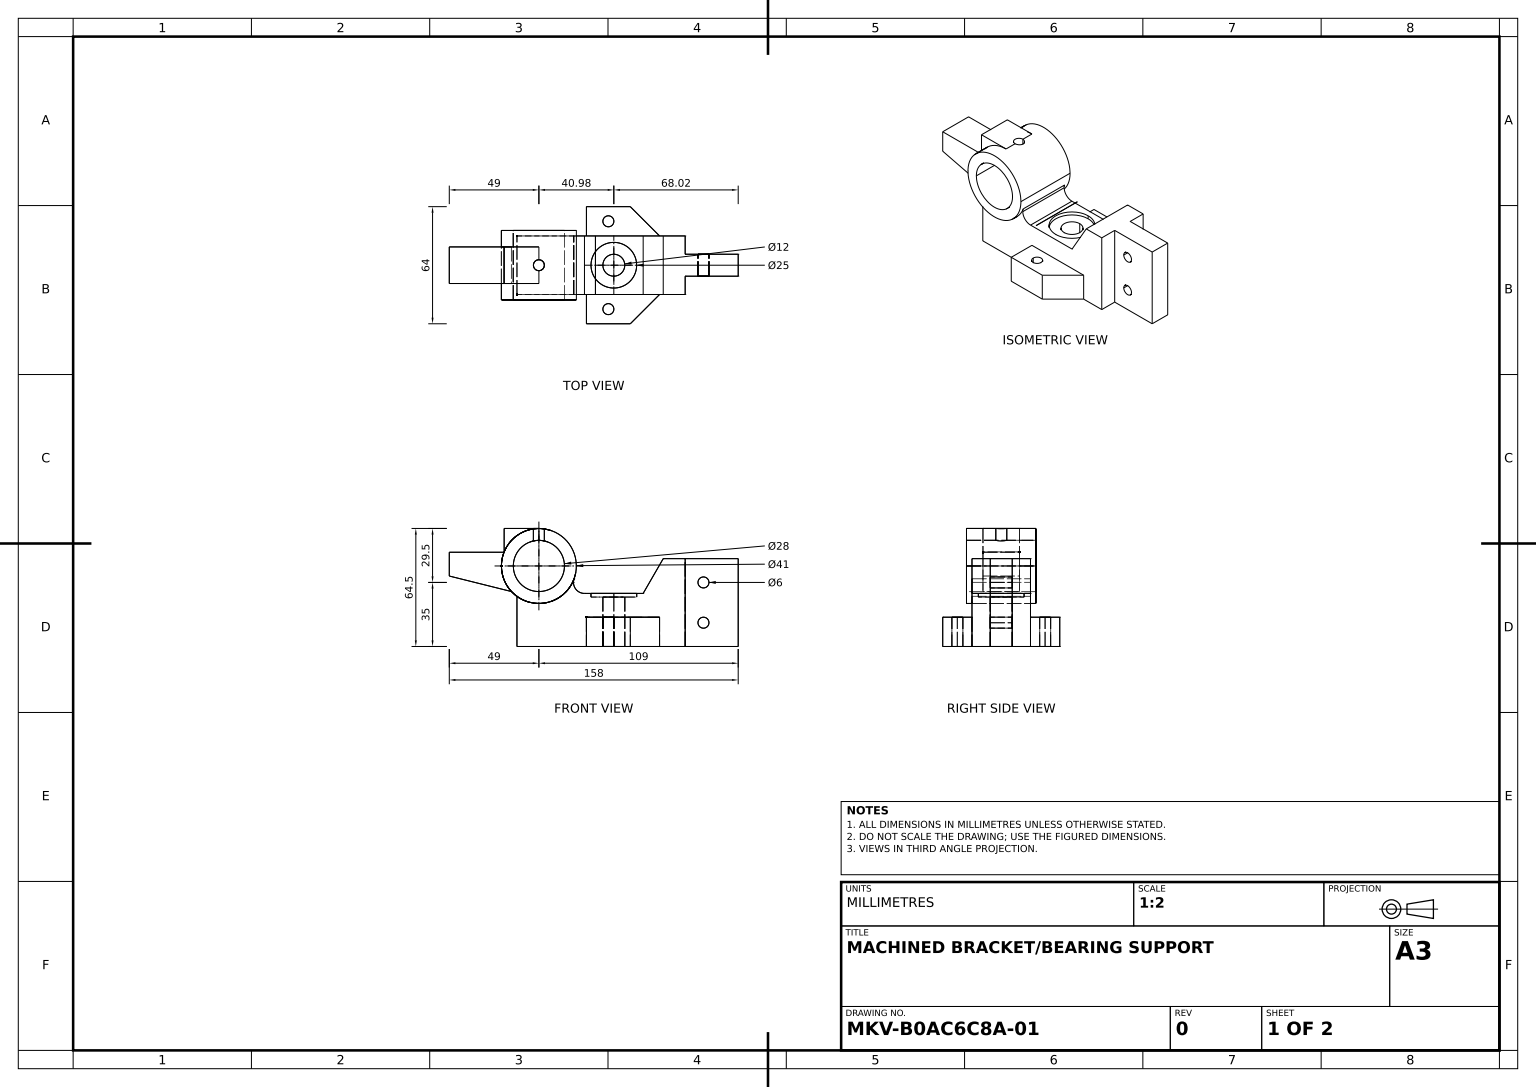
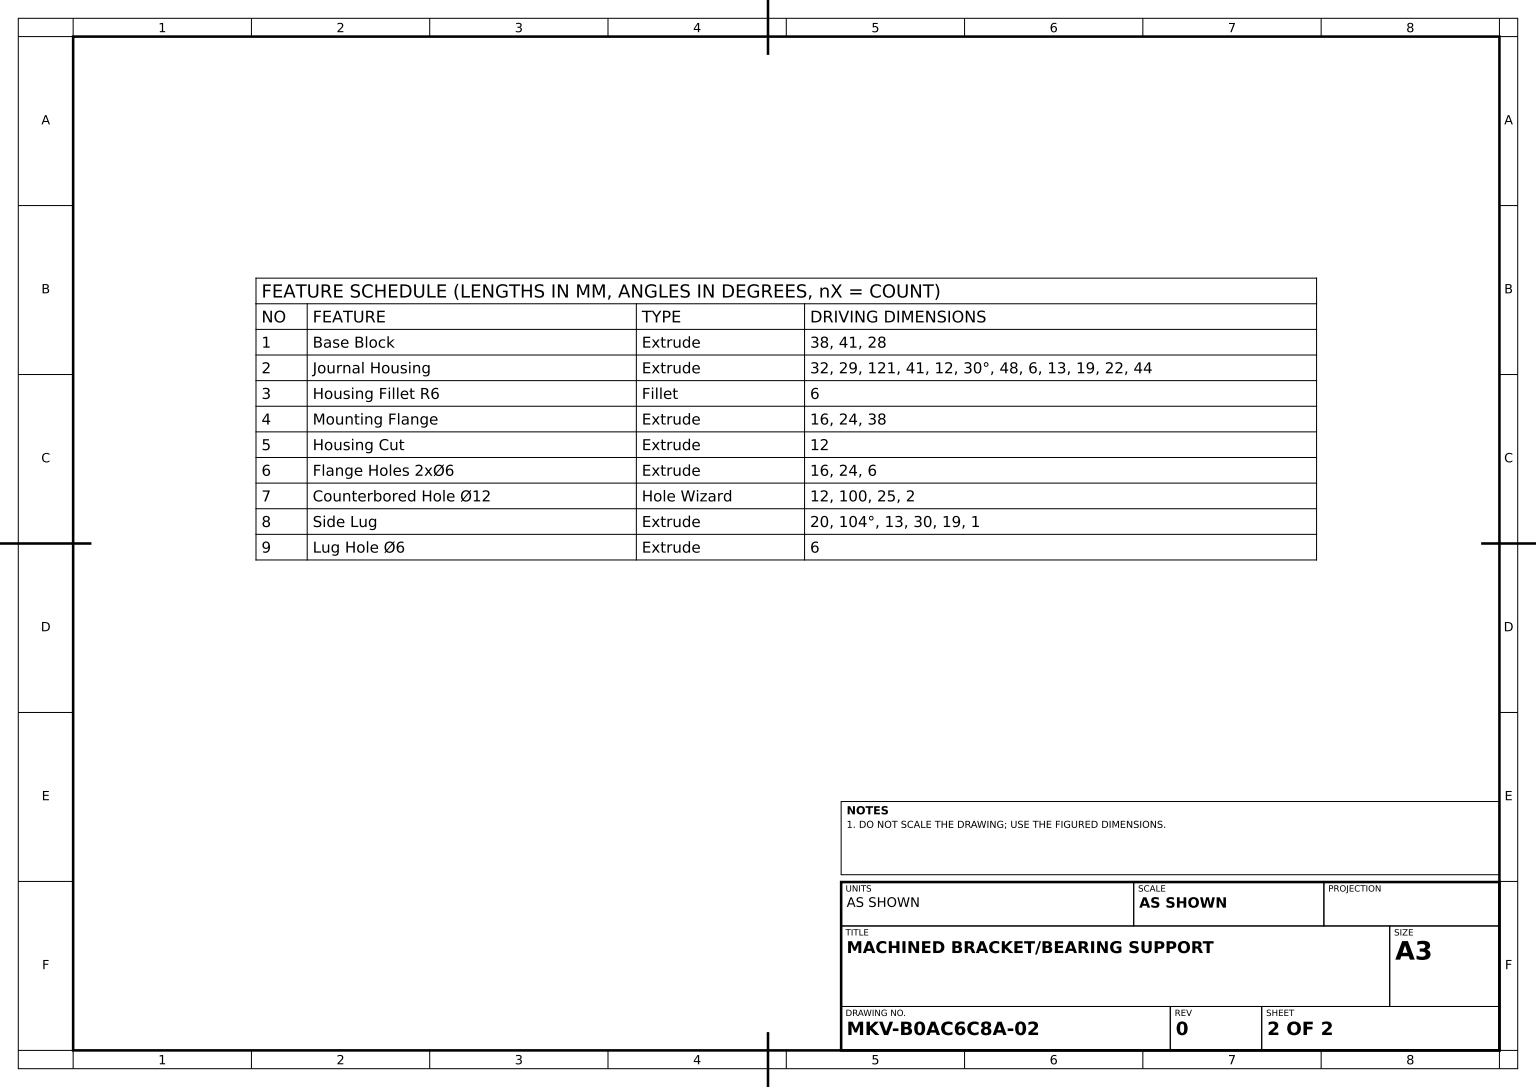
SolidWorks part; units mm, degrees
material "Plain Carbon Steel"
ref_plane "Front Plane" through (0, 0, 0) normal (0, 0, 1) x (1, 0, 0)
ref_plane "Top Plane" through (0, 0, 0) normal (0, 1, 0) x (1, 0, 0)
ref_plane "Right Plane" through (0, 0, 0) normal (1, 0, 0) x (0, 0, -1)
sketch "Base Block Sketch" plane through (0, 0, 0) normal (0, 0, 1) x (1, 0, 0)
  circle A0 centre (0, 0) radius 20.5
  circle A1 centre (0, 0) radius 14
  dimension "D1" = 41
  dimension "D2" = 28
extrude "Base Block" add sketch "Base Block Sketch" along normal mid plane 38
sketch "Journal Housing Profile Sketch" plane through (0, 0, 0) normal (0, 0, 1) x (1, 0, 0)
  line L0 (-12, -44) -> (-12, -15)
  line L1 (-12, -15) -> (57.0303, -15)
  line L2 (57.0303, -15) -> (68, 4)
  line L3 (68, 4) -> (109, 4)
  line L4 (109, 4) -> (109, -44)
  line L5 (109, -44) -> (-12, -44)
  line L6 (80, 4) -> (80, -34.5035) construction
  circle A1 centre (90, -31) radius 3
  circle A2 centre (90, -9) radius 3
  dimension "D8" = 6
  dimension "D1" = 29
  dimension "D2" = 121
  dimension "D3" = 41
  dimension "D4" = 12
  dimension "D5" = 30
  dimension "D6" = 44
  dimension "D7" = 48
  dimension "D9" = 13
  dimension "D10" = 19
  dimension "D11" = 22
  dimension "D12" = 12
extrude "Journal Housing" add sketch "Journal Housing Profile Sketch" along normal mid plane 32
fillet "Housing Fillet R6" radius 6 1 edges at (13.9732, -15, 0)
sketch "Mounting Flange Sketch" plane through (0, -44, 0) normal (0, -1, 0) x (1, 0, 0)
  line L0 (26, 16) -> (26, 32)
  line L1 (57.0303, 16) -> (24.9249, 16) construction
  line L2 (26, 32) -> (50, 32)
  line L3 (50, 32) -> (66, 16)
  line L4 (109, 16) -> (68, 16) construction
  line L5 (26, 16) -> (66, 16)
  line L7 (-12, 16) -> (-12, -16) construction
  line L8 (0, 0) -> (123.5825, 0) construction
  line L9 (50, -32) -> (66, -16)
  line L10 (26, -32) -> (50, -32)
  line L11 (26, -16) -> (66, -16)
  line L12 (26, -16) -> (26, -32)
  dimension "D1" = 16
  dimension "D2" = 24
  dimension "D3" = 16
  dimension "D4" = 38
extrude "Mounting Flange" add sketch "Mounting Flange Sketch" against normal blind 16
sketch "Housing Cut Sketch" plane through (0, 4, 0) normal (0, 1, 0) x (1, 0, 0)
  line L0 (68, -16) -> (68, 16) construction
  line L1 (109, -16) -> (80, -16)
  line L2 (109, -16) -> (109, -6)
  line L3 (109, -6) -> (80, -6)
  line L4 (80, -16) -> (80, -6)
  line L5 (109, 16) -> (80, 16)
  line L6 (109, 16) -> (109, 6)
  line L7 (109, 6) -> (80, 6)
  line L8 (80, 16) -> (80, 6)
  dimension "D1" = 12
  dimension "D2" = 12
extrude "Housing Cut" cut sketch "Housing Cut Sketch" against normal through all
sketch "Flange Holes Sketch" plane through (0, -28, 0) normal (0, 1, 0) x (1, 0, 0)
  line L0 (0, 0) -> (18.2916, 0) construction
  line L1 (50, -32) -> (26, -32) construction
  circle A0 centre (38, -24) radius 3
  circle A1 centre (38, 24) radius 3
  point P7 (38, -32)
  dimension "D2" = 6
  dimension "D1" = 24
extrude "Flange Holes 2xØ6" cut sketch "Flange Holes Sketch" against normal blind 16
hole_wizard "Counterbored Hole Ø12" positions "3DSketch1" profile "Sketch8" legacy
sketch3d "3DSketch1"
  line L1 (24.9249, -15, 0) -> (56.6013, -15, 0) construction
  line L2 (24.9249, -15, -16) -> (24.9249, -15, 16) construction
  line L5 (40.9776, -15, 16) -> (40.9776, -15, -16) construction
  line L6 (57.0303, -15, 16) -> (24.9249, -15, 16) construction
  line L7 (57.0303, -15, -16) -> (24.9249, -15, -16) construction
  point P0 (40.9776, -15, 0)
sketch "Sketch8" plane through (40.9776, -15, 0) normal (1, 0, 0) x (0, 0, 1)
  line L0 (0, 0) -> (0, 99.7885)
  line L1 (0, 99.7885) -> (6, 99.7885)
  line L2 (6, 99.7885) -> (6, 2)
  line L3 (6, 2) -> (12.5, 2)
  line L4 (12.5, 2) -> (12.5, 0)
  line L5 (12.5, 0) -> (0, 0)
  line L6 (0, 110) -> (0, -10) construction
  dimension "Diameter" = 12
  dimension "Depth" = 100
  dimension "C-Bore Diameter" = 25
  dimension "C-Bore Depth" = 2
sketch "Side Lug Sketch" plane through (0, 0, 0) normal (0, 0, 1) x (1, 0, 0)
  line L0 (0, 20.5) -> (-19, 20.5)
  line L2 (-19, 7.5) -> (-49, 7.5)
  line L3 (-49, 7.5) -> (-49, -5.5)
  line L4 (-49, -5.5) -> (-13.0901, -14.4533)
  line L5 (-19, 20.5) -> (-19, 7.5)
  line L6 (0, 20.5) -> (0, 19.5)
  circle A2 centre (0, 0) radius 20.5 construction
  circle A4 centre (0, 0) radius 19.5
  arc A5 (0, 19.5) -> (-13.0901, -14.4533) centre (0, 0) ccw
  dimension "D1" = 104
  dimension "D2" = 13
  dimension "D3" = 19
  dimension "D4" = 30
  dimension "D5" = 13
  dimension "D6" = 1
extrude "Side Lug" add sketch "Side Lug Sketch" along normal mid plane 20
sketch "Lug Hole Sketch" plane through (0, 20.5, 0) normal (0, 1, 0) x (1, 0, 0)
  circle A0 centre (0, 0) radius 3
  dimension "D1" = 6
extrude "Lug Hole Ø6" cut sketch "Lug Hole Sketch" against normal up to next
